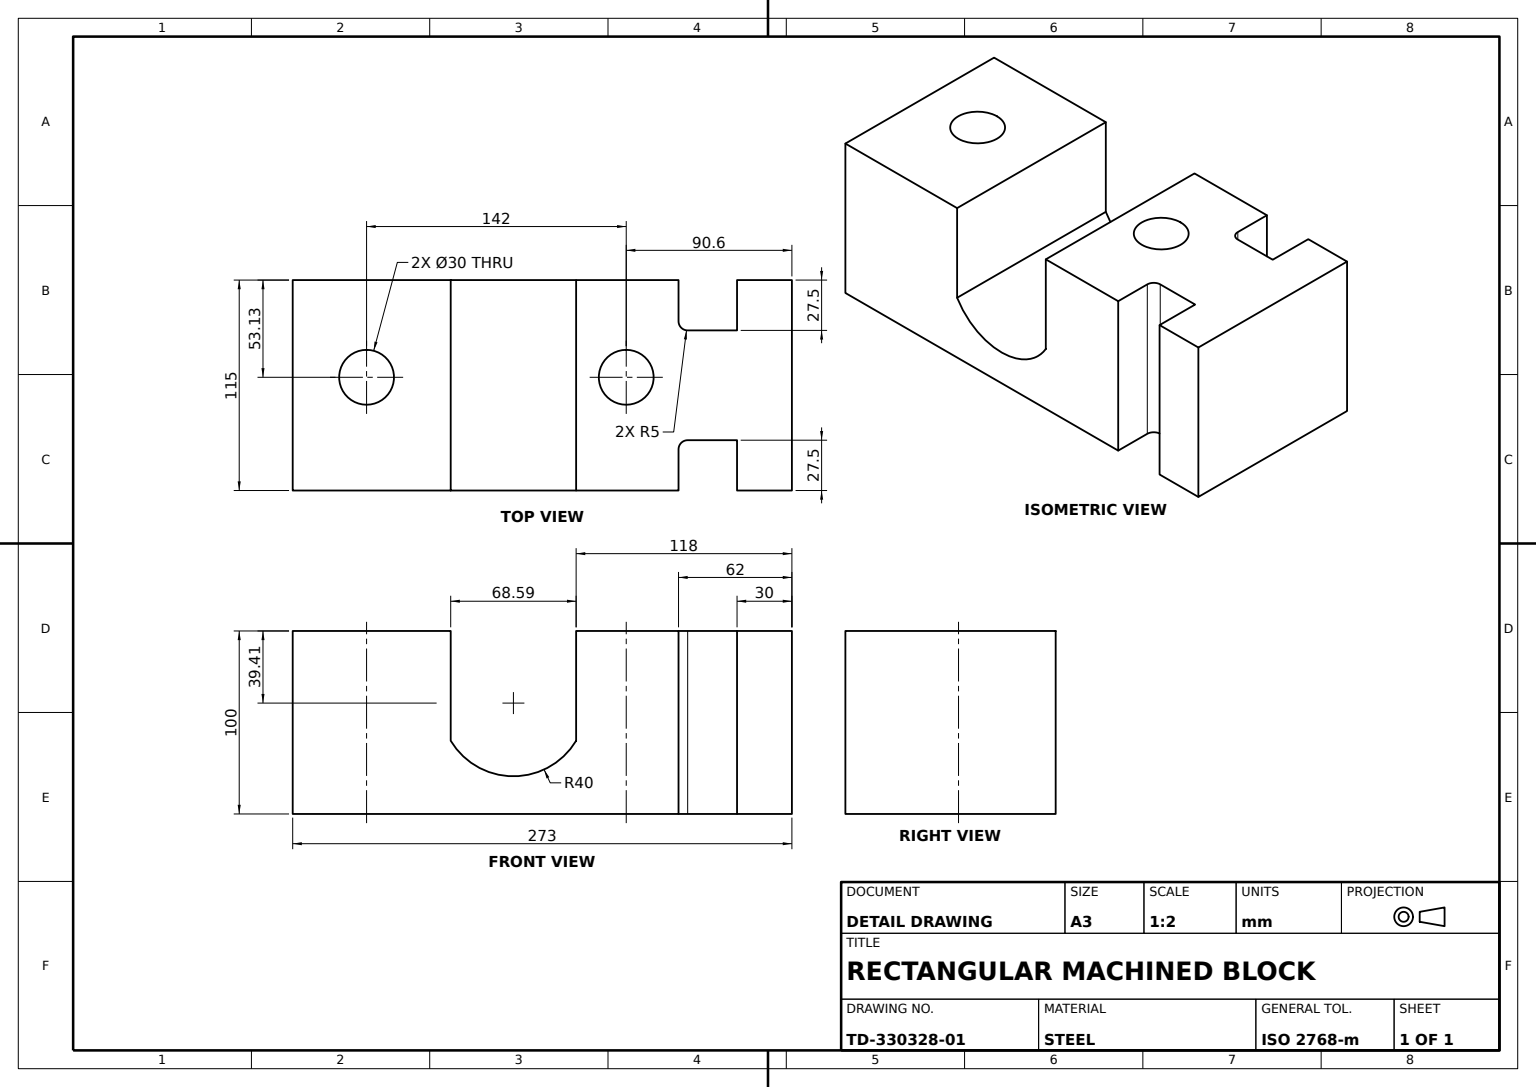
from build123d import *

# Parameters (mm, degrees)
SUPPORT_PROFILE_SKETCH_W         = 115
SUPPORT_PROFILE_SKETCH_H         = 30
SUPPORT_BODY_DEPTH               = 100
SIDE_MOUNTING_HOLES_SKETCH_R     = 15
SIDE_MOUNTING_HOLES_2X_DEPTH     = 324.8628221
OPEN_BEARING_SEAT_CUT_DEPTH      = 324.8628221
OPEN_BEARING_SEAT_CUT_DEPTH_BACK = 324.8628221


with BuildPart() as part:
    # Support Profile Sketch → Support Body (new body)
    with BuildSketch(Plane.XY):
        with BuildLine():
            Line((27.5, 57), (27.5, 30))
            Line((27.5, 30), (57.5, 30))
            Line((57.5, 30), (87.5, 30))
            Line((87.5, 30), (87.5, 57))
            ThreePointArc((87.5, 57), (88.964466094, 60.535533906), (92.5, 62))
            Line((92.5, 62), (115, 62))
            Line((115, 62), (115, 273))
            ThreePointArc((115, 273), (57.5, 285.765861395), (0, 273))
            Line((0, 273), (0, 62))
            Line((0, 62), (22.5, 62))
            ThreePointArc((22.5, 62), (26.035533906, 60.535533906), (27.5, 57))
        make_face()
        with Locations((57.5, 15)):
            Rectangle(SUPPORT_PROFILE_SKETCH_W, SUPPORT_PROFILE_SKETCH_H)
    extrude(amount=SUPPORT_BODY_DEPTH)

    # Side Mounting Holes Sketch → Side Mounting Holes 2x (cut, through all)
    with BuildSketch(Plane.XY.offset(100)):
        with Locations((53.126487568, 232.599577538)):
            Circle(SIDE_MOUNTING_HOLES_SKETCH_R)
        with Locations((53.126487568, 90.599577538)):
            Circle(SIDE_MOUNTING_HOLES_SKETCH_R)
    extrude(amount=-SIDE_MOUNTING_HOLES_2X_DEPTH, mode=Mode.SUBTRACT)

    # Bearing Seat Sketch → Open Bearing Seat Cut (cut, two sides: drawn at the far end of the back side and taken through both)
    with BuildSketch(Plane.ZY.offset(-OPEN_BEARING_SEAT_CUT_DEPTH_BACK)):
        with BuildLine():
            Line((-500.188374916, 118), (0, 118))
            Line((0, 118), (60, 118))
            ThreePointArc((60, 118), (79.41198533, 152.294805029), (60, 186.589610057))
            Line((60, 186.589610057), (0, 186.589610057))
            Line((0, 186.589610057), (0, 273))
            Line((0, 273), (100, 273))
            Line((100, 273), (100, 180.5))
            Line((100, 180.5), (108, 180.5))
            Line((108, 180.5), (108, 135.5))
            Line((108, 135.5), (100, 135.5))
            Line((100, 135.5), (100, 62))
            Line((100, 62), (100, -438.188374916))
            Line((100, -438.188374916), (779.965669758, 295.569302764))
            Line((779.965669758, 295.569302764), (179.777294842, 851.75767768))
            Line((179.777294842, 851.75767768), (-500.188374916, 118))
        make_face()
    extrude(amount=OPEN_BEARING_SEAT_CUT_DEPTH + OPEN_BEARING_SEAT_CUT_DEPTH_BACK, mode=Mode.SUBTRACT)


solid = part.part
